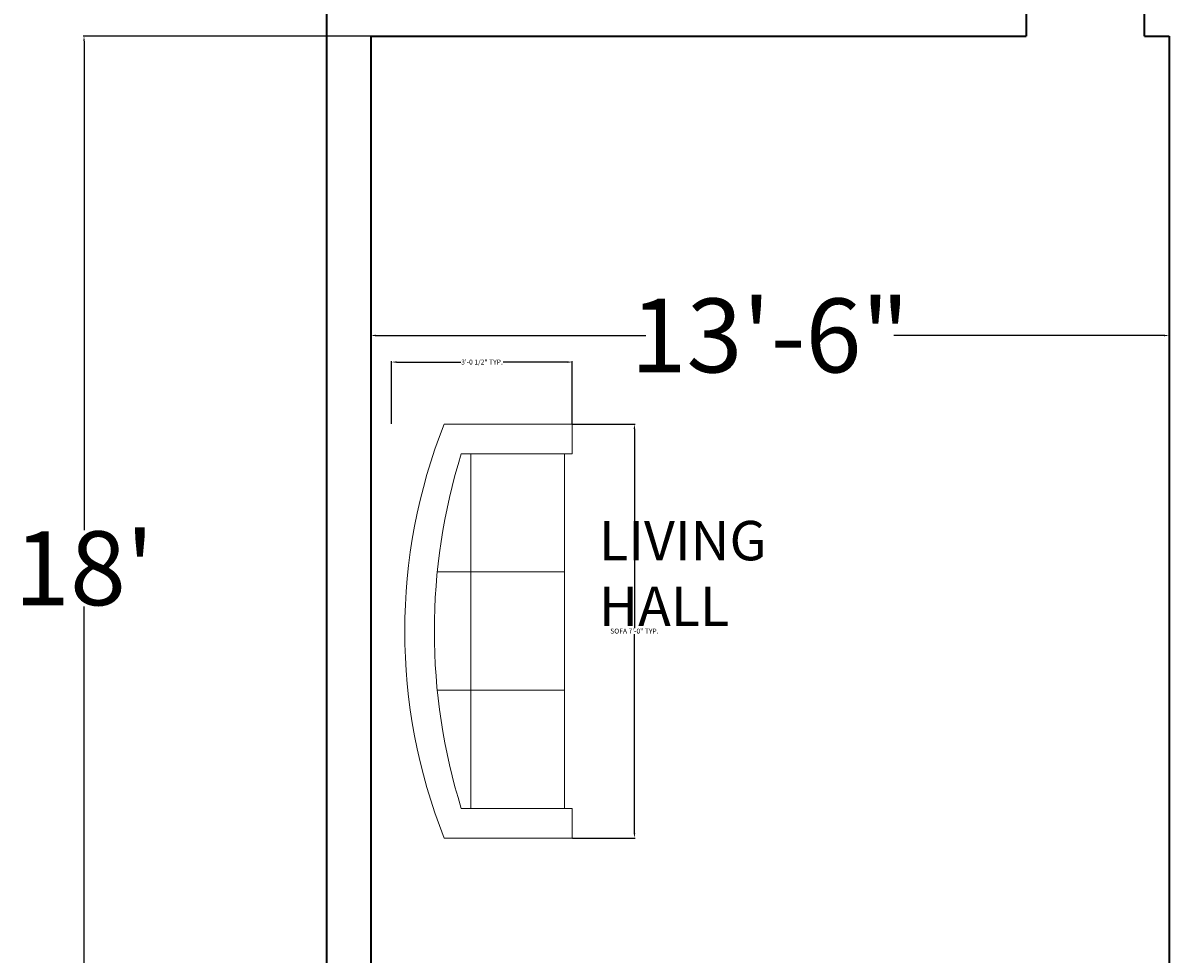
# Model space of a CAD drawing. Units: inches. Extents: x 371 to 1095, y -45 to 1219.
# Tile 9 of 18: x 431 to 664, y 610 to 799. Entities that reach past the tile are written whole.
import ezdxf

# ---------------------------------------------------------------- set-up
doc = ezdxf.new("R2010")
doc.units = ezdxf.units.IN
doc.header["$MEASUREMENT"] = 0
for name, color, linetype, lineweight in [('A-ANNO-DIMS', 2, 'Continuous', 18), ('A-AREA-IDEN', 7, 'Continuous', 18), ('A-FURN', 254, 'Continuous', 18), ('A-WALL', 40, 'Continuous', 35)]:
    doc.layers.add(name, color=color, linetype=linetype, lineweight=lineweight)
doc.styles.get("Standard").update_dxf_attribs({"font": 'arial.ttf'})
doc.dimstyles.get("Standard").update_dxf_attribs({"dimtxt": 1, "dimasz": 1, "dimexe": 0.18, "dimexo": 0.0625, "dimgap": 0.09, "dimtad": 0, "dimtih": 1, "dimtoh": 1, "dimdec": 0, "dimzin": 0, "dimdsep": 46, "dimlunit": 3, "dimtxsty": 'Standard', "dimcen": 0.09, "dimadec": 0, "dimazin": 0, "dimtfac": 1, "dimtdec": 0, "dimtofl": 0, "dimtmove": 0, "dimatfit": 3, "dimfxl": 1, "dimtolj": 1, "dimtzin": 0, "dimarcsym": 0})

# ---------------------------------------------------------------- blocks, each defined once
blk = doc.blocks.new('Sofa - Roundback 7 ft.')
for p, q in [((-12.00002, -32.4421), (-12.00003, -6.5971)), ((11.99997, -32.4421), (11.99998, -6.5971)), ((-36.000027, -34), (-36.000027, -11.4696)), ((35.99998, -34), (35.99998, -11.4696)), ((-35.999844, -13.3819), (35.9998, -13.3819)), ((-36.000027, -32.4421), (35.99998, -32.4421))]:
    blk.add_line(p, q)
for points in [[(-36.000027, -34), (-42.000027, -34), (-42.000027, -8)], [(41.99998, -8), (41.99998, -34), (35.99998, -34)]]:
    blk.add_lwpolyline(points)
for centre, radius, start, end in [((0, -114.25), 114.25, 68.43141, 111.5686), ((-0.00001, -127.1968), 121.1968, 72.72033, 107.2797)]:
    blk.add_arc(centre, radius, start, end)
blk = doc.blocks.new('*D20')
at = {"layer": 'A-ANNO-DIMS', "color": 0, "lineweight": -2, "transparency": 16777216}
for p, q in [((501.75, 796.03), (443.44, 796.03)), ((443.62, 795.03), (443.62, 695.77)), ((443.62, 581.03), (443.62, 680.28)), ((501.75, 580.03), (443.44, 580.03))]:
    blk.add_line(p, q, dxfattribs=at)
at = {"layer": 'A-ANNO-DIMS', "color": 0, "transparency": 16777216}
for points in [[(443.46, 795.03), (443.79, 795.03), (443.62, 796.03)], [(443.46, 581.03), (443.79, 581.03), (443.62, 580.03)]]:
    blk.add_solid(points, dxfattribs=at)
at = {"layer": 'Defpoints', "color": 0, "transparency": 16777216}
for p in [(501.81, 796.03), (443.62, 580.03), (501.81, 580.03)]:
    blk.add_point(p, dxfattribs=at)
at = {"layer": 'A-ANNO-DIMS', "color": 0, "transparency": 16777216, "insert": (443.62, 688.03), "char_height": 1, "attachment_point": 5}
blk.add_mtext("\\A1;{\\H15x;18'}", dxfattribs=at)
blk = doc.blocks.new('*D22')
at = {"layer": 'A-ANNO-DIMS', "color": 0, "lineweight": -2, "transparency": 16777216}
for p, q in [((501.81, 795.96), (501.81, 735.1)), ((663.81, 795.96), (663.81, 735.1)), ((502.81, 735.28), (557.66, 735.28)), ((662.81, 735.28), (607.96, 735.28))]:
    blk.add_line(p, q, dxfattribs=at)
at = {"layer": 'A-ANNO-DIMS', "color": 0, "transparency": 16777216}
for points in [[(502.81, 735.44), (502.81, 735.11), (501.81, 735.28)], [(662.81, 735.44), (662.81, 735.11), (663.81, 735.28)]]:
    blk.add_solid(points, dxfattribs=at)
at = {"layer": 'Defpoints', "color": 0, "transparency": 16777216}
for p in [(501.81, 796.03), (663.81, 796.03), (663.81, 735.28)]:
    blk.add_point(p, dxfattribs=at)
at = {"layer": 'A-ANNO-DIMS', "color": 0, "transparency": 16777216, "insert": (582.81, 735.28), "char_height": 1, "attachment_point": 5}
blk.add_mtext('\\A1;{\\H15x;13\'-6"}', dxfattribs=at)
blk = doc.blocks.new('*D32')
at = {"layer": 'A-ANNO-DIMS', "color": 0, "lineweight": -2, "transparency": 16777216}
for p, q in [((542.77, 717.28), (555.49, 717.28)), ((555.31, 716.28), (555.31, 675.88)), ((555.31, 634.28), (555.31, 674.67)), ((542.77, 633.28), (555.49, 633.28))]:
    blk.add_line(p, q, dxfattribs=at)
at = {"layer": 'A-ANNO-DIMS', "color": 0, "transparency": 16777216}
for points in [[(555.15, 716.28), (555.48, 716.28), (555.31, 717.28)], [(555.15, 634.28), (555.48, 634.28), (555.31, 633.28)]]:
    blk.add_solid(points, dxfattribs=at)
at = {"layer": 'Defpoints', "color": 0, "transparency": 16777216}
for p in [(542.71, 717.28), (555.31, 717.28), (542.71, 633.28)]:
    blk.add_point(p, dxfattribs=at)
at = {"layer": 'A-ANNO-DIMS', "color": 0, "transparency": 16777216, "insert": (555.31, 675.28), "char_height": 1, "attachment_point": 5}
blk.add_mtext('\\A1;SOFA 7\'-0" TYP.', dxfattribs=at)
blk = doc.blocks.new('*D33')
at = {"layer": 'A-ANNO-DIMS', "color": 0, "lineweight": -2, "transparency": 16777216}
for p, q in [((506.05, 717.34), (506.05, 730.06)), ((507.05, 729.88), (520.08, 729.88)), ((541.71, 729.88), (528.68, 729.88)), ((542.71, 717.34), (542.71, 730.06))]:
    blk.add_line(p, q, dxfattribs=at)
at = {"layer": 'A-ANNO-DIMS', "color": 0, "transparency": 16777216}
for points in [[(507.05, 730.04), (507.05, 729.71), (506.05, 729.88)], [(541.71, 730.04), (541.71, 729.71), (542.71, 729.88)]]:
    blk.add_solid(points, dxfattribs=at)
at = {"layer": 'Defpoints', "color": 0, "transparency": 16777216}
for p in [(506.05, 729.88), (506.05, 717.28), (542.71, 717.28)]:
    blk.add_point(p, dxfattribs=at)
at = {"layer": 'A-ANNO-DIMS', "color": 0, "transparency": 16777216, "insert": (524.38, 729.88), "char_height": 1, "attachment_point": 5}
blk.add_mtext('\\A1;3\'-0 1/2" TYP.', dxfattribs=at)

msp = doc.modelspace()

# ---------------------------------------------------------------- linework, layer by layer
at = {"layer": 'A-WALL'}
for p, q in [((492.81, 982.03), (492.81, 82.03)), ((634.81, 805.03), (634.81, 796.03)), ((658.81, 796.03), (658.81, 805.03)), ((501.81, 796.03), (634.81, 796.03)), ((501.81, 796.03), (501.81, 580.03)), ((658.81, 796.03), (663.81, 796.03)), ((663.81, 796.03), (663.81, 451.03))]:
    msp.add_line(p, q, dxfattribs=at)

# ---------------------------------------------------------------- block references
at = {"layer": 'A-FURN', "rotation": 90}
msp.add_blockref('Sofa - Roundback 7 ft.', (508.71, 675.28), dxfattribs=at)

# ---------------------------------------------------------------- texts
at = {"layer": 'A-AREA-IDEN', "insert": (548.12, 697.64), "char_height": 8, "attachment_point": 1}
msp.add_mtext_dynamic_manual_height_columns('LIVING HALL', width=53.6318, gutter_width=1, heights=[0], dxfattribs=at)

# ---------------------------------------------------------------- dimensions: what is measured, and where the dimension line sits
at = {"layer": 'A-ANNO-DIMS'}
for base, p1, p2, angle, text, override, picture, middle in [((443.62, 580.03), (501.81, 796.03), (501.81, 580.03), 90, '{\\H15x;<>}', {"dimclrd": 0, "dimclre": 0, "dimclrt": 0}, '*D20', (443.62, 688.03)), ((506.05, 729.88), (542.71, 717.28), (506.05, 717.28), 180, '<> TYP.', {"dimdec": 1, "dimlfac": 1, "dimrnd": 0, "dimzin": 1, "dimdsep": 46, "dimlunit": 4, "dimfrac": 2}, '*D33', (524.38, 729.88)), ((555.31, 717.28), (542.71, 633.28), (542.71, 717.28), 90, 'SOFA <> TYP.', {"dimdec": 1, "dimlfac": 1, "dimrnd": 0, "dimzin": 1, "dimdsep": 46, "dimlunit": 4, "dimfrac": 2}, '*D32', (555.31, 675.28))]:
    dim = msp.add_linear_dim(base=base, p1=p1, p2=p2, angle=angle, text=text, dimstyle='Standard', override=override, dxfattribs=at)
    dim.commit()
    dim.dimension.update_dxf_attribs({"geometry": picture, "text_midpoint": middle})
dim = msp.add_linear_dim(base=(663.81, 735.28), p1=(501.81, 796.03), p2=(663.81, 796.03), text='{\\H15x;<>}', dimstyle='Standard', override={"dimclrd": 0, "dimclre": 0, "dimclrt": 0}, dxfattribs=at)
dim.commit()
dim.dimension.update_dxf_attribs({"geometry": '*D22', "text_midpoint": (582.81, 735.28)})

doc.saveas('drawing.dxf')
